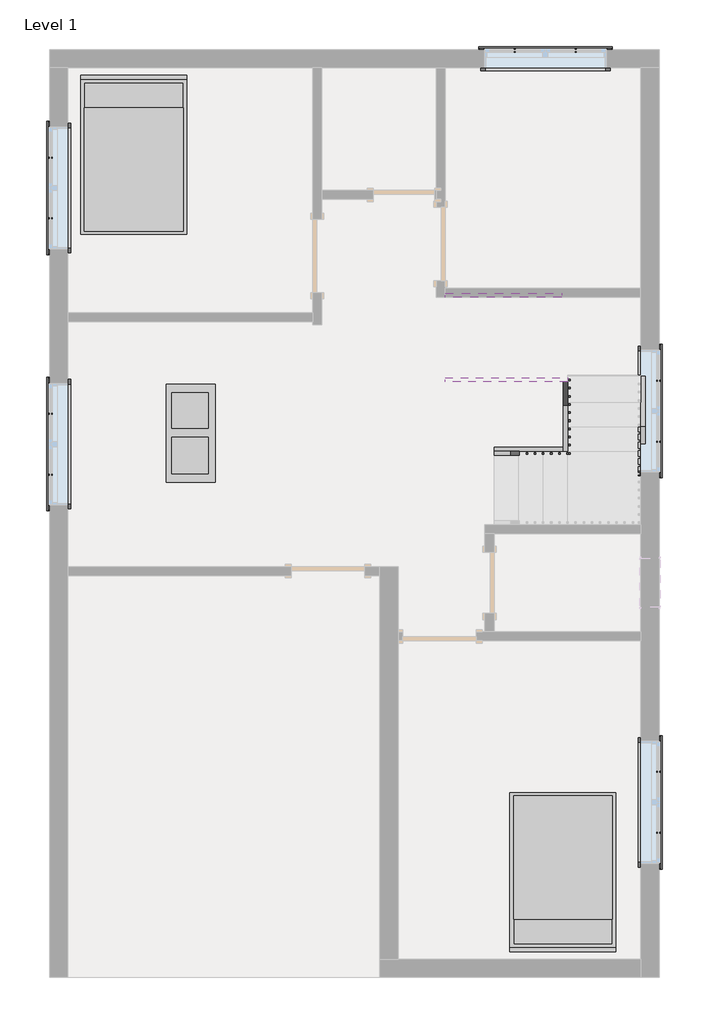
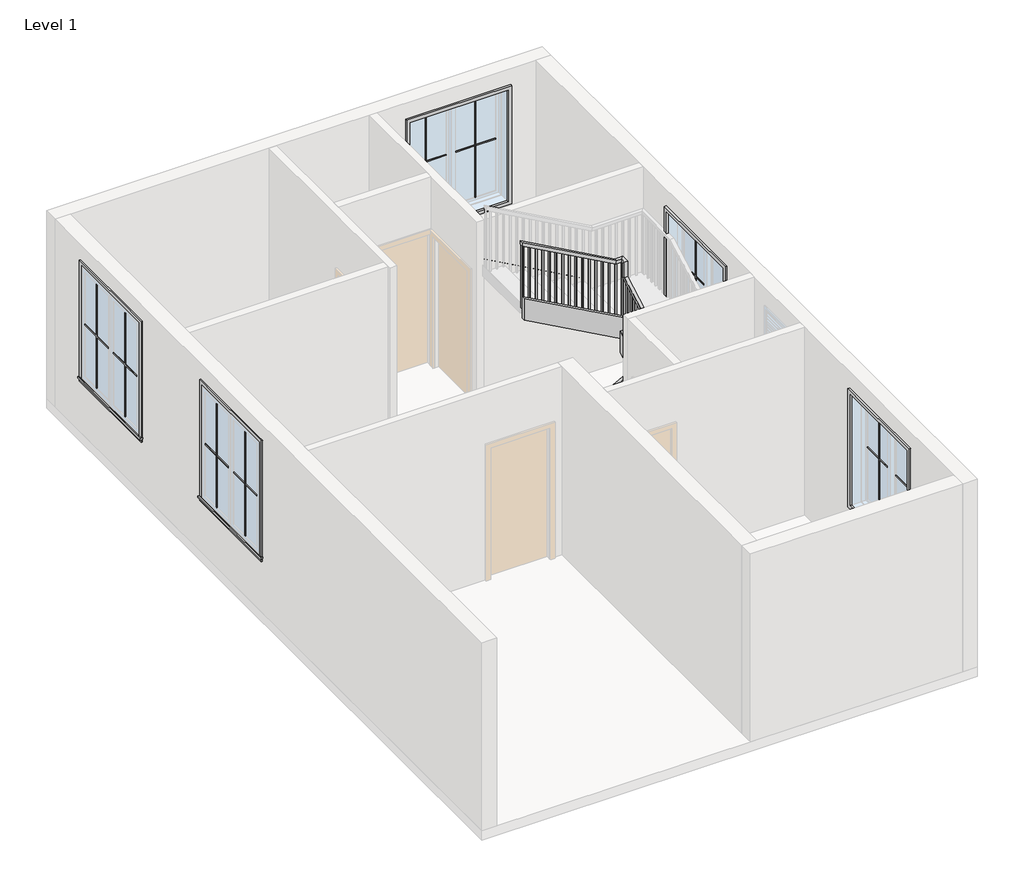
# One storey, part 2 of 2: 21 proxies, 6 members, 2 furniture elements, 1 railing.
"""IFC4 building model written with IfcOpenShell, lengths in millimetres."""

from ifc_helpers import new_model, si_unit, frame, origin, place, context, project, spatial, polyline, outline, extrude, faceted_brep, transform, mapped, element, save
from components import muntin_pattern_2x2_muntin_pattern_2x2_f6a80940, muntin_pattern_2x2_muntin_pattern_2x2_09b00a1c, trim_window_exterior_flat_with_sill_698ed857, trim_window_interior_flat_picture_frame_92551a5e, coffee_table_with_brass_mullions_11320_coffee_table_with_5962bef7, bed_17739_bed_17739_15c61121

model = new_model("IFC4")

# Units and contexts
model_context = context("Model", 3, world=origin())
ifc_project = project(units=[si_unit("LENGTHUNIT", "METRE", prefix="MILLI")], contexts=[model_context])

# Site, building, storey
site = spatial("IfcSite", under=ifc_project)
building = spatial("IfcBuilding", under=site)
storey = spatial("IfcBuildingStorey", under=building, Name="Level 1", Elevation=0.0)

# Proxies
placement = place(None, origin())
muntin_pattern_2x2_muntin_pattern_2x2_shape = muntin_pattern_2x2_muntin_pattern_2x2_f6a80940(model_context)
element("IfcBuildingElementProxy", 1, Name="Muntin Pattern_2x2 : Muntin Pattern_2x2", ObjectType="Muntin Pattern_2x2 : Muntin Pattern_2x2", at=placement, inside=storey, context=model_context, shape_type="MappedRepresentation", body=[
    mapped(muntin_pattern_2x2_muntin_pattern_2x2_shape, transform((-4589.1575206, 441.8004493, 984.25), x_axis=(0.0, 1.0, 0.0), y_axis=(-1.0, 0.0, 0.0), z_axis=(0.0, 0.0, 1.0))),
])
element("IfcBuildingElementProxy", 2, Name="Muntin Pattern_2x2 : Muntin Pattern_2x2", ObjectType="Muntin Pattern_2x2 : Muntin Pattern_2x2", at=placement, inside=storey, context=model_context, shape_type="MappedRepresentation", body=[
    mapped(muntin_pattern_2x2_muntin_pattern_2x2_shape, transform((-4589.1575206, 3632.6754493, 984.25), x_axis=(0.0, 1.0, 0.0), y_axis=(-1.0, 0.0, 0.0), z_axis=(0.0, 0.0, 1.0))),
])
element("IfcBuildingElementProxy", 3, Name="Muntin Pattern_2x2 : Muntin Pattern_2x2", ObjectType="Muntin Pattern_2x2 : Muntin Pattern_2x2", at=placement, inside=storey, context=model_context, shape_type="MappedRepresentation", body=[
    mapped(muntin_pattern_2x2_muntin_pattern_2x2_shape, transform((1197.2799794, 5726.5879493, 984.25), x_axis=(1.0, 0.0, 0.0), y_axis=(0.0, 1.0, 0.0), z_axis=(0.0, 0.0, 1.0))),
])
element("IfcBuildingElementProxy", 4, Name="Muntin Pattern_2x2 : Muntin Pattern_2x2", ObjectType="Muntin Pattern_2x2 : Muntin Pattern_2x2", at=placement, inside=storey, context=model_context, shape_type="MappedRepresentation", body=[
    mapped(muntin_pattern_2x2_muntin_pattern_2x2_shape, transform((2986.3924794, 1613.3754493, 984.25), x_axis=(0.0, -1.0, 0.0), y_axis=(1.0, 0.0, 0.0), z_axis=(0.0, 0.0, 1.0))),
])
element("IfcBuildingElementProxy", 5, Name="Muntin Pattern_2x2 : Muntin Pattern_2x2", ObjectType="Muntin Pattern_2x2 : Muntin Pattern_2x2", at=placement, inside=storey, context=model_context, shape_type="MappedRepresentation", body=[
    mapped(muntin_pattern_2x2_muntin_pattern_2x2_shape, transform((2986.3924794, -3260.2495507, 984.25), x_axis=(0.0, -1.0, 0.0), y_axis=(1.0, 0.0, 0.0), z_axis=(0.0, 0.0, 1.0))),
])
muntin_pattern_2x2_muntin_pattern_2x2_2_shape = muntin_pattern_2x2_muntin_pattern_2x2_09b00a1c(model_context)
element("IfcBuildingElementProxy", 6, Name="Muntin Pattern_2x2 : Muntin Pattern_2x2", ObjectType="Muntin Pattern_2x2 : Muntin Pattern_2x2", at=placement, inside=storey, context=model_context, shape_type="MappedRepresentation", body=[
    mapped(muntin_pattern_2x2_muntin_pattern_2x2_2_shape, transform((-4589.1575206, 1200.6254493, 984.25), x_axis=(0.0, -1.0, 0.0), y_axis=(1.0, 0.0, 0.0), z_axis=(0.0, 0.0, 1.0))),
])
element("IfcBuildingElementProxy", 7, Name="Muntin Pattern_2x2 : Muntin Pattern_2x2", ObjectType="Muntin Pattern_2x2 : Muntin Pattern_2x2", at=placement, inside=storey, context=model_context, shape_type="MappedRepresentation", body=[
    mapped(muntin_pattern_2x2_muntin_pattern_2x2_2_shape, transform((-4589.1575206, 4391.5004493, 984.25), x_axis=(0.0, -1.0, 0.0), y_axis=(1.0, 0.0, 0.0), z_axis=(0.0, 0.0, 1.0))),
])
element("IfcBuildingElementProxy", 8, Name="Muntin Pattern_2x2 : Muntin Pattern_2x2", ObjectType="Muntin Pattern_2x2 : Muntin Pattern_2x2", at=placement, inside=storey, context=model_context, shape_type="MappedRepresentation", body=[
    mapped(muntin_pattern_2x2_muntin_pattern_2x2_2_shape, transform((1956.1049794, 5726.5879493, 984.25), x_axis=(-1.0, 0.0, 0.0), y_axis=(0.0, -1.0, 0.0), z_axis=(0.0, 0.0, 1.0))),
])
element("IfcBuildingElementProxy", 9, Name="Muntin Pattern_2x2 : Muntin Pattern_2x2", ObjectType="Muntin Pattern_2x2 : Muntin Pattern_2x2", at=placement, inside=storey, context=model_context, shape_type="MappedRepresentation", body=[
    mapped(muntin_pattern_2x2_muntin_pattern_2x2_2_shape, transform((2986.3924794, 854.5504493, 984.25), x_axis=(0.0, 1.0, 0.0), y_axis=(-1.0, 0.0, 0.0), z_axis=(0.0, 0.0, 1.0))),
])
element("IfcBuildingElementProxy", 10, Name="Muntin Pattern_2x2 : Muntin Pattern_2x2", ObjectType="Muntin Pattern_2x2 : Muntin Pattern_2x2", at=placement, inside=storey, context=model_context, shape_type="MappedRepresentation", body=[
    mapped(muntin_pattern_2x2_muntin_pattern_2x2_2_shape, transform((2986.3924794, -4019.0745507, 984.25), x_axis=(0.0, 1.0, 0.0), y_axis=(-1.0, 0.0, 0.0), z_axis=(0.0, 0.0, 1.0))),
])
trim_window_exterior_flat_with_sill_shape = trim_window_exterior_flat_with_sill_698ed857(model_context)
element("IfcBuildingElementProxy", 11, Name="Trim-Window-Exterior-Flat : with Sill", ObjectType="Trim-Window-Exterior-Flat : with Sill", at=placement, inside=storey, context=model_context, shape_type="MappedRepresentation", body=[
    mapped(trim_window_exterior_flat_with_sill_shape, transform((-4598.6825206, 821.2129493, 2743.2), x_axis=(0.0, -1.0, 0.0), y_axis=(0.0, 0.0, 1.0), z_axis=(-1.0, 0.0, 0.0))),
])
element("IfcBuildingElementProxy", 12, Name="Trim-Window-Exterior-Flat : with Sill", ObjectType="Trim-Window-Exterior-Flat : with Sill", at=placement, inside=storey, context=model_context, shape_type="MappedRepresentation", body=[
    mapped(trim_window_exterior_flat_with_sill_shape, transform((-4598.6825206, 4012.0879493, 2743.2), x_axis=(0.0, -1.0, 0.0), y_axis=(0.0, 0.0, 1.0), z_axis=(-1.0, 0.0, 0.0))),
])
element("IfcBuildingElementProxy", 13, Name="Trim-Window-Exterior-Flat : with Sill", ObjectType="Trim-Window-Exterior-Flat : with Sill", at=placement, inside=storey, context=model_context, shape_type="MappedRepresentation", body=[
    mapped(trim_window_exterior_flat_with_sill_shape, transform((1576.6924794, 5736.1129493, 2743.2), x_axis=(-1.0, 0.0, 0.0), y_axis=(0.0, 0.0, 1.0), z_axis=(0.0, 1.0, 0.0))),
])
element("IfcBuildingElementProxy", 14, Name="Trim-Window-Exterior-Flat : with Sill", ObjectType="Trim-Window-Exterior-Flat : with Sill", at=placement, inside=storey, context=model_context, shape_type="MappedRepresentation", body=[
    mapped(trim_window_exterior_flat_with_sill_shape, transform((2995.9174794, 1233.9629493, 2743.2), x_axis=(0.0, 1.0, 0.0), y_axis=(0.0, 0.0, 1.0), z_axis=(1.0, 0.0, 0.0))),
])
element("IfcBuildingElementProxy", 15, Name="Trim-Window-Exterior-Flat : with Sill", ObjectType="Trim-Window-Exterior-Flat : with Sill", at=placement, inside=storey, context=model_context, shape_type="MappedRepresentation", body=[
    mapped(trim_window_exterior_flat_with_sill_shape, transform((2995.9174794, -3639.6620507, 2743.2), x_axis=(0.0, 1.0, 0.0), y_axis=(0.0, 0.0, 1.0), z_axis=(1.0, 0.0, 0.0))),
])
trim_window_interior_flat_picture_frame_shape = trim_window_interior_flat_picture_frame_92551a5e(model_context)
element("IfcBuildingElementProxy", 16, Name="Trim-Window-Interior-Flat : Picture Frame", ObjectType="Trim-Window-Interior-Flat : Picture Frame", at=placement, inside=storey, context=model_context, shape_type="MappedRepresentation", body=[
    mapped(trim_window_interior_flat_picture_frame_shape, transform((-4370.0825206, 821.2129493, 2743.2), x_axis=(0.0, 1.0, 0.0), y_axis=(0.0, 0.0, 1.0), z_axis=(1.0, 0.0, 0.0))),
])
element("IfcBuildingElementProxy", 17, Name="Trim-Window-Interior-Flat : Picture Frame", ObjectType="Trim-Window-Interior-Flat : Picture Frame", at=placement, inside=storey, context=model_context, shape_type="MappedRepresentation", body=[
    mapped(trim_window_interior_flat_picture_frame_shape, transform((-4370.0825206, 4012.0879493, 2743.2), x_axis=(0.0, 1.0, 0.0), y_axis=(0.0, 0.0, 1.0), z_axis=(1.0, 0.0, 0.0))),
])
element("IfcBuildingElementProxy", 18, Name="Trim-Window-Interior-Flat : Picture Frame", ObjectType="Trim-Window-Interior-Flat : Picture Frame", at=placement, inside=storey, context=model_context, shape_type="MappedRepresentation", body=[
    mapped(trim_window_interior_flat_picture_frame_shape, transform((1576.6924794, 5507.5129493, 2743.2), x_axis=(1.0, 0.0, 0.0), y_axis=(0.0, 0.0, 1.0), z_axis=(0.0, -1.0, 0.0))),
])
element("IfcBuildingElementProxy", 19, Name="Trim-Window-Interior-Flat : Picture Frame", ObjectType="Trim-Window-Interior-Flat : Picture Frame", at=placement, inside=storey, context=model_context, shape_type="MappedRepresentation", body=[
    mapped(trim_window_interior_flat_picture_frame_shape, transform((2767.3174794, 1233.9629493, 2743.2), x_axis=(0.0, -1.0, 0.0), y_axis=(0.0, 0.0, 1.0), z_axis=(-1.0, 0.0, 0.0))),
])
element("IfcBuildingElementProxy", 20, Name="Trim-Window-Interior-Flat : Picture Frame", ObjectType="Trim-Window-Interior-Flat : Picture Frame", at=placement, inside=storey, context=model_context, shape_type="MappedRepresentation", body=[
    mapped(trim_window_interior_flat_picture_frame_shape, transform((2767.3174794, -3639.6620507, 2743.2), x_axis=(0.0, -1.0, 0.0), y_axis=(0.0, 0.0, 1.0), z_axis=(-1.0, 0.0, 0.0))),
])
coffee_table_with_brass_mullions_11320_coffee_table_with_shape = coffee_table_with_brass_mullions_11320_coffee_table_with_5962bef7(model_context)
element("IfcBuildingElementProxy", 21, Name="coffee_table_with_brass_mullions_11320 : coffee_table_with_brass_mullions_11320", ObjectType="coffee_table_with_brass_mullions_11320 : coffee_table_with_brass_mullions_11320", at=placement, inside=storey, context=model_context, shape_type="MappedRepresentation", body=[
    mapped(coffee_table_with_brass_mullions_11320_coffee_table_with_shape, transform((-2412.0418112, 1596.9678033, 0.0), x_axis=(0.0, 1.0, 0.0), y_axis=(-1.0, 0.0, 0.0), z_axis=(0.0, 0.0, 1.0))),
])

# Furniture
bed_17739_bed_17739_shape = bed_17739_bed_17739_15c61121(model_context)
element("IfcFurniture", 22, ObjectType="Bed_17739 : Bed_17739", at=placement, inside=storey, context=model_context, shape_type="MappedRepresentation", body=[
    mapped(bed_17739_bed_17739_shape, transform((-3550.9325206, 4402.6129493, 0.0), x_axis=(1.0, 0.0, 0.0), y_axis=(0.0, 1.0, 0.0), z_axis=(0.0, 0.0, 1.0))),
])
element("IfcFurniture", 23, ObjectType="Bed_17739 : Bed_17739", at=placement, inside=storey, context=model_context, shape_type="MappedRepresentation", body=[
    mapped(bed_17739_bed_17739_shape, transform((1795.7674794, -4487.3870507, 0.0), x_axis=(-1.0, 0.0, 0.0), y_axis=(0.0, -1.0, 0.0), z_axis=(0.0, 0.0, 1.0))),
])

# Members
element("IfcMember", 24, ObjectType="Stringer - 2\" Width", at=placement, inside=storey, context=model_context, shape_type="SweptSolid", body=[
    extrude(outline(polyline([(207.5983948, 938.5174794), (0.0, 938.5174794), (0.0, 1192.4619822), (338.6974984, 1802.1174794), (687.3761726, 1802.1174794), (207.5983948, 938.5174794)])), frame((0.0, 732.3129493, 0.0), z_axis=(0.0, 1.0, 0.0), x_axis=(0.0, 0.0, 1.0)), (0.0, 0.0, 1.0), 50.8),
])
element("IfcMember", 25, ObjectType="Stringer - 2\" Width", at=placement, inside=storey, context=model_context, shape_type="SweptSolid", body=[
    extrude(outline(polyline([(732.3129493, 536.253054), (732.3129493, 884.9317281), (1595.9129493, 1364.7095059), (1595.9129493, 1016.0308318), (732.3129493, 536.253054)])), frame((1802.1174794, 0.0, 0.0), z_axis=(1.0, 0.0, 0.0), x_axis=(0.0, 1.0, 0.0)), (0.0, 0.0, 1.0), 50.8),
])
element("IfcMember", 26, ObjectType="Stringer - 2\" Width", at=placement, inside=storey, context=model_context, shape_type="SweptSolid", body=[
    extrude(outline(polyline([(1213.5863873, 1852.9174794), (1562.2650614, 1852.9174794), (2408.9317281, 328.9174794), (2060.253054, 328.9174794), (1213.5863873, 1852.9174794)])), frame((0.0, 1595.9129493, 0.0), z_axis=(0.0, 1.0, 0.0), x_axis=(0.0, 0.0, 1.0)), (0.0, 0.0, 1.0), 50.8),
])
element("IfcMember", 27, ObjectType="Stringer - 2\" Width", at=placement, inside=storey, context=model_context, shape_type="SweptSolid", body=[
    extrude(outline(polyline([(207.5983948, 938.5174794), (0.0, 938.5174794), (0.0, 1192.4619822), (376.9317281, 1870.9390928), (376.9317281, 1243.3174794), (207.5983948, 938.5174794)])), frame((0.0, -232.8870507, 0.0), z_axis=(0.0, 1.0, 0.0), x_axis=(0.0, 0.0, 1.0)), (0.0, 0.0, 1.0), 50.8),
])
element("IfcMember", 28, ObjectType="Stringer - 2\" Width", at=placement, inside=storey, context=model_context, shape_type="SweptSolid", body=[
    extrude(outline(polyline([(714.2913359, 874.9197207), (1037.1129493, 1054.2650614), (1664.7345627, 1054.2650614), (1341.9129493, 874.9197207), (714.2913359, 874.9197207)])), frame((2767.3174794, 0.0, 0.0), z_axis=(1.0, 0.0, 0.0), x_axis=(0.0, 1.0, 0.0)), (0.0, 0.0, 1.0), 50.8),
])
element("IfcMember", 29, ObjectType="Stringer - 2\" Width", at=placement, inside=storey, context=model_context, shape_type="SweptSolid", body=[
    extrude(outline(polyline([(1601.6419429, 1782.0390928), (2408.9317281, 328.9174794), (2060.253054, 328.9174794), (1601.6419429, 1154.4174794), (1601.6419429, 1782.0390928)])), frame((0.0, 2650.0129493, 0.0), z_axis=(0.0, 1.0, 0.0), x_axis=(0.0, 0.0, 1.0)), (0.0, 0.0, 1.0), 50.8),
])

# Railing
element("IfcRailing", 30, ObjectType="Handrail - Rectangular", at=placement, inside=storey, context=model_context, shape_type="SolidModel", body=[
    faceted_brep([(938.5174794, 732.3129493, 1083.7333333), (938.5174794, 732.3129493, 1025.620221), (938.5174794, 681.5129493, 1025.620221), (938.5174794, 681.5129493, 1083.7333333), (1776.7174794, 732.3129493, 1549.4), (1827.5174794, 732.3129493, 1519.5091099), (1827.5174794, 681.5129493, 1519.5091099), (1776.7174794, 681.5129493, 1549.4), (1776.7174794, 732.3129493, 1803.4), (1827.5174794, 732.3129493, 1752.6), (1827.5174794, 681.5129493, 1752.6), (1776.7174794, 681.5129493, 1803.4), (1852.9174794, 732.3129493, 1803.4), (1852.9174794, 732.3129493, 1752.6), (1903.7174794, 681.5129493, 1752.6), (1903.7174794, 681.5129493, 1803.4), (1852.9174794, 808.5129493, 1803.4), (1852.9174794, 821.6765516, 1752.6), (1903.7174794, 821.6765516, 1752.6), (1903.7174794, 808.5129493, 1803.4), (1852.9174794, 1570.5129493, 2226.7333333), (1852.9174794, 1621.3129493, 2196.8424432), (1903.7174794, 1621.3129493, 2196.8424432), (1903.7174794, 1570.5129493, 2226.7333333), (1852.9174794, 1570.5129493, 2480.7333333), (1852.9174794, 1621.3129493, 2429.9333333), (1903.7174794, 1621.3129493, 2429.9333333), (1903.7174794, 1570.5129493, 2480.7333333), (1852.9174794, 1646.7129493, 2480.7333333), (1852.9174794, 1646.7129493, 2429.9333333), (1903.7174794, 1697.5129493, 2429.9333333), (1903.7174794, 1697.5129493, 2480.7333333), (1776.7174794, 1646.7129493, 2480.7333333), (1763.5538772, 1646.7129493, 2429.9333333), (1763.5538772, 1697.5129493, 2429.9333333), (1776.7174794, 1697.5129493, 2480.7333333), (328.9174794, 1646.7129493, 3285.0666667), (328.9174794, 1697.5129493, 3285.0666667), (328.9174794, 1697.5129493, 3226.9535543), (328.9174794, 1646.7129493, 3226.9535543)], [[[0, 1, 2, 3]], [[1, 0, 4, 5]], [[2, 1, 5, 6]], [[3, 2, 6, 7]], [[0, 3, 7, 4]], [[5, 4, 8, 9]], [[6, 5, 9, 10]], [[7, 6, 10, 11]], [[4, 7, 11, 8]], [[9, 8, 12, 13]], [[10, 9, 13, 14]], [[11, 10, 14, 15]], [[8, 11, 15, 12]], [[13, 12, 16, 17]], [[14, 13, 17, 18]], [[15, 14, 18, 19]], [[12, 15, 19, 16]], [[17, 16, 20, 21]], [[18, 17, 21, 22]], [[19, 18, 22, 23]], [[16, 19, 23, 20]], [[21, 20, 24, 25]], [[22, 21, 25, 26]], [[23, 22, 26, 27]], [[20, 23, 27, 24]], [[25, 24, 28, 29]], [[26, 25, 29, 30]], [[27, 26, 30, 31]], [[24, 27, 31, 28]], [[29, 28, 32, 33]], [[30, 29, 33, 34]], [[31, 30, 34, 35]], [[28, 31, 35, 32]], [[36, 37, 38, 39]], [[33, 32, 36, 39]], [[34, 33, 39, 38]], [[35, 34, 38, 37]], [[32, 35, 37, 36]]]),
    extrude(outline(polyline([(3218.1341099, 344.7924794), (2201.3333333, 344.7924794), (2201.3333333, 363.8424794), (3207.5507765, 363.8424794), (3218.1341099, 344.7924794)])), frame((0.0, 1662.5879493, 0.0), z_axis=(0.0, 1.0, 0.0), x_axis=(0.0, 0.0, 1.0)), (0.0, 0.0, 1.0), 19.05),
    extrude(outline(polyline([(3161.6896654, 446.3924794), (2201.3333333, 446.3924794), (2201.3333333, 465.4424794), (3151.1063321, 465.4424794), (3161.6896654, 446.3924794)])), frame((0.0, 1662.5879493, 0.0), z_axis=(0.0, 1.0, 0.0), x_axis=(0.0, 0.0, 1.0)), (0.0, 0.0, 1.0), 19.05),
    extrude(outline(polyline([(3105.245221, 547.9924794), (2201.3333333, 547.9924794), (2201.3333333, 567.0424794), (3094.6618876, 567.0424794), (3105.245221, 547.9924794)])), frame((0.0, 1662.5879493, 0.0), z_axis=(0.0, 1.0, 0.0), x_axis=(0.0, 0.0, 1.0)), (0.0, 0.0, 1.0), 19.05),
    extrude(outline(polyline([(3048.8007765, 649.5924794), (2032.0, 649.5924794), (2032.0, 668.6424794), (3038.2174432, 668.6424794), (3048.8007765, 649.5924794)])), frame((0.0, 1662.5879493, 0.0), z_axis=(0.0, 1.0, 0.0), x_axis=(0.0, 0.0, 1.0)), (0.0, 0.0, 1.0), 19.05),
    extrude(outline(polyline([(2992.3563321, 751.1924794), (2032.0, 751.1924794), (2032.0, 770.2424794), (2981.7729988, 770.2424794), (2992.3563321, 751.1924794)])), frame((0.0, 1662.5879493, 0.0), z_axis=(0.0, 1.0, 0.0), x_axis=(0.0, 0.0, 1.0)), (0.0, 0.0, 1.0), 19.05),
    extrude(outline(polyline([(2935.9118876, 852.7924794), (2032.0, 852.7924794), (2032.0, 871.8424794), (2925.3285543, 871.8424794), (2935.9118876, 852.7924794)])), frame((0.0, 1662.5879493, 0.0), z_axis=(0.0, 1.0, 0.0), x_axis=(0.0, 0.0, 1.0)), (0.0, 0.0, 1.0), 19.05),
    extrude(outline(polyline([(2879.4674432, 954.3924794), (1862.6666667, 954.3924794), (1862.6666667, 973.4424794), (2868.8841099, 973.4424794), (2879.4674432, 954.3924794)])), frame((0.0, 1662.5879493, 0.0), z_axis=(0.0, 1.0, 0.0), x_axis=(0.0, 0.0, 1.0)), (0.0, 0.0, 1.0), 19.05),
    extrude(outline(polyline([(2823.0229988, 1055.9924794), (1862.6666667, 1055.9924794), (1862.6666667, 1075.0424794), (2812.4396654, 1075.0424794), (2823.0229988, 1055.9924794)])), frame((0.0, 1662.5879493, 0.0), z_axis=(0.0, 1.0, 0.0), x_axis=(0.0, 0.0, 1.0)), (0.0, 0.0, 1.0), 19.05),
    extrude(outline(polyline([(2766.5785543, 1157.5924794), (1862.6666667, 1157.5924794), (1862.6666667, 1176.6424794), (2755.995221, 1176.6424794), (2766.5785543, 1157.5924794)])), frame((0.0, 1662.5879493, 0.0), z_axis=(0.0, 1.0, 0.0), x_axis=(0.0, 0.0, 1.0)), (0.0, 0.0, 1.0), 19.05),
    extrude(outline(polyline([(2710.1341099, 1259.1924794), (1693.3333333, 1259.1924794), (1693.3333333, 1278.2424794), (2699.5507765, 1278.2424794), (2710.1341099, 1259.1924794)])), frame((0.0, 1662.5879493, 0.0), z_axis=(0.0, 1.0, 0.0), x_axis=(0.0, 0.0, 1.0)), (0.0, 0.0, 1.0), 19.05),
    extrude(outline(polyline([(2653.6896654, 1360.7924794), (1693.3333333, 1360.7924794), (1693.3333333, 1379.8424794), (2643.1063321, 1379.8424794), (2653.6896654, 1360.7924794)])), frame((0.0, 1662.5879493, 0.0), z_axis=(0.0, 1.0, 0.0), x_axis=(0.0, 0.0, 1.0)), (0.0, 0.0, 1.0), 19.05),
    extrude(outline(polyline([(2597.245221, 1462.3924794), (1693.3333333, 1462.3924794), (1693.3333333, 1481.4424794), (2586.6618876, 1481.4424794), (2597.245221, 1462.3924794)])), frame((0.0, 1662.5879493, 0.0), z_axis=(0.0, 1.0, 0.0), x_axis=(0.0, 0.0, 1.0)), (0.0, 0.0, 1.0), 19.05),
    extrude(outline(polyline([(2540.8007765, 1563.9924794), (1524.0, 1563.9924794), (1524.0, 1583.0424794), (2530.2174432, 1583.0424794), (2540.8007765, 1563.9924794)])), frame((0.0, 1662.5879493, 0.0), z_axis=(0.0, 1.0, 0.0), x_axis=(0.0, 0.0, 1.0)), (0.0, 0.0, 1.0), 19.05),
    extrude(outline(polyline([(2484.3563321, 1665.5924794), (1524.0, 1665.5924794), (1524.0, 1684.6424794), (2473.7729988, 1684.6424794), (2484.3563321, 1665.5924794)])), frame((0.0, 1662.5879493, 0.0), z_axis=(0.0, 1.0, 0.0), x_axis=(0.0, 0.0, 1.0)), (0.0, 0.0, 1.0), 19.05),
    extrude(outline(polyline([(2427.9118876, 1767.1924794), (1524.0, 1767.1924794), (1524.0, 1786.2424794), (2417.3285543, 1786.2424794), (2427.9118876, 1767.1924794)])), frame((0.0, 1662.5879493, 0.0), z_axis=(0.0, 1.0, 0.0), x_axis=(0.0, 0.0, 1.0)), (0.0, 0.0, 1.0), 19.05),
    extrude(outline(polyline([(1868.7924794, 1611.7879493), (1868.7924794, 1630.8379493), (1887.8424794, 1630.8379493), (1887.8424794, 1611.7879493), (1868.7924794, 1611.7879493)])), frame((0.0, 0.0, 1185.3333333), z_axis=(0.0, 0.0, 1.0), x_axis=(1.0, 0.0, 0.0)), (0.0, 0.0, 1.0), 1244.6),
    extrude(outline(polyline([(1529.2379493, 2145.6896654), (1529.2379493, 1185.3333333), (1510.1879493, 1185.3333333), (1510.1879493, 2135.1063321), (1529.2379493, 2145.6896654)])), frame((1868.7924794, 0.0, 0.0), z_axis=(1.0, 0.0, 0.0), x_axis=(0.0, 1.0, 0.0)), (0.0, 0.0, 1.0), 19.05),
    extrude(outline(polyline([(1427.6379493, 2089.245221), (1427.6379493, 1185.3333333), (1408.5879493, 1185.3333333), (1408.5879493, 2078.6618876), (1427.6379493, 2089.245221)])), frame((1868.7924794, 0.0, 0.0), z_axis=(1.0, 0.0, 0.0), x_axis=(0.0, 1.0, 0.0)), (0.0, 0.0, 1.0), 19.05),
    extrude(outline(polyline([(1326.0379493, 2032.8007765), (1326.0379493, 1016.0), (1306.9879493, 1016.0), (1306.9879493, 2022.2174432), (1326.0379493, 2032.8007765)])), frame((1868.7924794, 0.0, 0.0), z_axis=(1.0, 0.0, 0.0), x_axis=(0.0, 1.0, 0.0)), (0.0, 0.0, 1.0), 19.05),
    extrude(outline(polyline([(1224.4379493, 1976.3563321), (1224.4379493, 1016.0), (1205.3879493, 1016.0), (1205.3879493, 1965.7729988), (1224.4379493, 1976.3563321)])), frame((1868.7924794, 0.0, 0.0), z_axis=(1.0, 0.0, 0.0), x_axis=(0.0, 1.0, 0.0)), (0.0, 0.0, 1.0), 19.05),
    extrude(outline(polyline([(1122.8379493, 1919.9118876), (1122.8379493, 1016.0), (1103.7879493, 1016.0), (1103.7879493, 1909.3285543), (1122.8379493, 1919.9118876)])), frame((1868.7924794, 0.0, 0.0), z_axis=(1.0, 0.0, 0.0), x_axis=(0.0, 1.0, 0.0)), (0.0, 0.0, 1.0), 19.05),
    extrude(outline(polyline([(1021.2379493, 1863.4674432), (1021.2379493, 846.6666667), (1002.1879493, 846.6666667), (1002.1879493, 1852.8841099), (1021.2379493, 1863.4674432)])), frame((1868.7924794, 0.0, 0.0), z_axis=(1.0, 0.0, 0.0), x_axis=(0.0, 1.0, 0.0)), (0.0, 0.0, 1.0), 19.05),
    extrude(outline(polyline([(919.6379493, 1807.0229988), (919.6379493, 846.6666667), (900.5879493, 846.6666667), (900.5879493, 1796.4396654), (919.6379493, 1807.0229988)])), frame((1868.7924794, 0.0, 0.0), z_axis=(1.0, 0.0, 0.0), x_axis=(0.0, 1.0, 0.0)), (0.0, 0.0, 1.0), 19.05),
    extrude(outline(polyline([(818.0379493, 1750.5785543), (818.0379493, 846.6666667), (798.9879493, 846.6666667), (798.9879493, 1739.995221), (818.0379493, 1750.5785543)])), frame((1868.7924794, 0.0, 0.0), z_axis=(1.0, 0.0, 0.0), x_axis=(0.0, 1.0, 0.0)), (0.0, 0.0, 1.0), 19.05),
    extrude(outline(polyline([(1843.3924794, 716.4379493), (1862.4424794, 716.4379493), (1862.4424794, 697.3879493), (1843.3924794, 697.3879493), (1843.3924794, 716.4379493)])), frame((0.0, 0.0, 677.3333333), z_axis=(0.0, 0.0, 1.0), x_axis=(1.0, 0.0, 0.0)), (0.0, 0.0, 1.0), 1075.2666667),
    extrude(outline(polyline([(1471.8841099, 1741.7924794), (508.0, 1741.7924794), (508.0, 1760.8424794), (1482.4674432, 1760.8424794), (1471.8841099, 1741.7924794)])), frame((0.0, 697.3879493, 0.0), z_axis=(0.0, 1.0, 0.0), x_axis=(0.0, 0.0, 1.0)), (0.0, 0.0, 1.0), 19.05),
    extrude(outline(polyline([(1415.4396654, 1640.1924794), (508.0, 1640.1924794), (508.0, 1659.2424794), (1426.0229988, 1659.2424794), (1415.4396654, 1640.1924794)])), frame((0.0, 697.3879493, 0.0), z_axis=(0.0, 1.0, 0.0), x_axis=(0.0, 0.0, 1.0)), (0.0, 0.0, 1.0), 19.05),
    extrude(outline(polyline([(1358.995221, 1538.5924794), (508.0, 1538.5924794), (508.0, 1557.6424794), (1369.5785543, 1557.6424794), (1358.995221, 1538.5924794)])), frame((0.0, 697.3879493, 0.0), z_axis=(0.0, 1.0, 0.0), x_axis=(0.0, 0.0, 1.0)), (0.0, 0.0, 1.0), 19.05),
    extrude(outline(polyline([(1302.5507765, 1436.9924794), (338.6666667, 1436.9924794), (338.6666667, 1456.0424794), (1313.1341099, 1456.0424794), (1302.5507765, 1436.9924794)])), frame((0.0, 697.3879493, 0.0), z_axis=(0.0, 1.0, 0.0), x_axis=(0.0, 0.0, 1.0)), (0.0, 0.0, 1.0), 19.05),
    extrude(outline(polyline([(1246.1063321, 1335.3924794), (338.6666667, 1335.3924794), (338.6666667, 1354.4424794), (1256.6896654, 1354.4424794), (1246.1063321, 1335.3924794)])), frame((0.0, 697.3879493, 0.0), z_axis=(0.0, 1.0, 0.0), x_axis=(0.0, 0.0, 1.0)), (0.0, 0.0, 1.0), 19.05),
    extrude(outline(polyline([(1189.6618876, 1233.7924794), (338.6666667, 1233.7924794), (338.6666667, 1252.8424794), (1200.245221, 1252.8424794), (1189.6618876, 1233.7924794)])), frame((0.0, 697.3879493, 0.0), z_axis=(0.0, 1.0, 0.0), x_axis=(0.0, 0.0, 1.0)), (0.0, 0.0, 1.0), 19.05),
    extrude(outline(polyline([(1133.2174432, 1132.1924794), (169.3333333, 1132.1924794), (169.3333333, 1151.2424794), (1143.8007765, 1151.2424794), (1133.2174432, 1132.1924794)])), frame((0.0, 697.3879493, 0.0), z_axis=(0.0, 1.0, 0.0), x_axis=(0.0, 0.0, 1.0)), (0.0, 0.0, 1.0), 19.05),
    extrude(outline(polyline([(1076.7729988, 1030.5924794), (169.3333333, 1030.5924794), (169.3333333, 1049.6424794), (1087.3563321, 1049.6424794), (1076.7729988, 1030.5924794)])), frame((0.0, 697.3879493, 0.0), z_axis=(0.0, 1.0, 0.0), x_axis=(0.0, 0.0, 1.0)), (0.0, 0.0, 1.0), 19.05),
    extrude(outline(polyline([(1868.7924794, 1662.5879493), (1868.7924794, 1681.6379493), (1887.8424794, 1681.6379493), (1887.8424794, 1662.5879493), (1868.7924794, 1662.5879493)])), frame((0.0, 0.0, 1354.6666667), z_axis=(0.0, 0.0, 1.0), x_axis=(1.0, 0.0, 0.0)), (0.0, 0.0, 1.0), 1075.2666667),
    extrude(outline(polyline([(1868.7924794, 716.4379493), (1887.8424794, 716.4379493), (1887.8424794, 697.3879493), (1868.7924794, 697.3879493), (1868.7924794, 716.4379493)])), frame((0.0, 0.0, 677.3333333), z_axis=(0.0, 0.0, 1.0), x_axis=(1.0, 0.0, 0.0)), (0.0, 0.0, 1.0), 1075.2666667),
    extrude(outline(polyline([(3226.9535543, 328.9174794), (2201.3333333, 328.9174794), (2201.3333333, 347.9674794), (3216.370221, 347.9674794), (3226.9535543, 328.9174794)])), frame((0.0, 1662.5879493, 0.0), z_axis=(0.0, 1.0, 0.0), x_axis=(0.0, 0.0, 1.0)), (0.0, 0.0, 1.0), 19.05),
    extrude(outline(polyline([(1025.620221, 938.5174794), (169.3333333, 938.5174794), (169.3333333, 957.5674794), (1036.2035543, 957.5674794), (1025.620221, 938.5174794)])), frame((0.0, 697.3879493, 0.0), z_axis=(0.0, 1.0, 0.0), x_axis=(0.0, 0.0, 1.0)), (0.0, 0.0, 1.0), 19.05),
])

save(model, "model.ifc")

# Revit data of these elements
# Type "Muntin Pattern_2x2 : Muntin Pattern_2x2"
#   Width [instance default] = 4' - 0"
#   Thickness = 0' - 0 1/2"
#   Height [instance default] = 4' - 0"
#   Distance = 0' - 0 3/4"
#   Interior Material [instance default] = none
#   Exterior Material [instance default] = none
#   Default Elevation = 0
# Type "Trim-Window-Exterior-Flat : with Sill"
#   Trim Width = 0' - 2 1/4"
#   Trim Thickness_Picture Frame = 0' - 1 1/4"
#   Trim Thickness_with Sill = 0' - 0 3/4"
#   Sill Thickness = 0' - 1 1/4"
#   Opening Width [instance default] = 2' - 0"
#   Opening Height [instance default] = 3' - 0"
#   Default Elevation = 4' - 0"
#   Sill = yes
#   Picture Frame = no
#   Trim Material [instance default] = none
# Type "Trim-Window-Interior-Flat : Picture Frame"
#   Trim Thickness_Picture Frame = 0' - 1 1/4"
#   Trim Width = 0' - 2 1/4"
#   Trim Thickness_with Sill = 0' - 0 3/4"
#   Sill Thickness = 0' - 1 1/4"
#   Opening Width [instance default] = 2' - 0"
#   Opening Height [instance default] = 3' - 0"
#   Default Elevation = 4' - 0"
#   Sill = no
#   Picture Frame = yes
#   Trim Material [instance default] = none
# Type "coffee_table_with_brass_mullions_11320 : coffee_table_with_brass_mullions_11320"
#   Default Elevation = 0
# Type "Bed_17739 : Bed_17739"
#   Default Elevation = 0
# Type "Handrail - Rectangular"
#   Assembly Code = "C2010400"
#   built-in parameter 1008612 = 0.0416667 (stored number, unit not read)
#   built-in parameter 1008611 = 0.0416667 (stored number, unit not read)
#   built-in parameter 1008609 = 0.333333 (stored number, unit not read)
#   built-in parameter 1008604 = 0.166667 (stored number, unit not read)
#   built-in parameter 1008603 = 0.166667 (stored number, unit not read)
#   Railing Height = 3' - 0"
#   built-in parameter 1008630 = 2
#   built-in parameter 1008610 = 2
#   built-in parameter 1008618 = Baluster - Square : 3/4"
# Elements 1, 2, 3, 4, 5, 6, 7, 8, 9, 10 (IfcBuildingElementProxy, "Muntin Pattern_2x2 : Muntin Pattern_2x2")
#   Width = 2' - 0 5/8"
#   Height = 5' - 6 1/2"
#   Interior Material = Wood - Stained
#   Exterior Material = Clad - White
#   Phase Created = New Construction
#   Materials on its faces: "Clad - White", "Wood - Stained"
# Elements 11, 12, 13, 14, 15 (IfcBuildingElementProxy, "Trim-Window-Exterior-Flat : with Sill")
#   Opening Width = 5' - 0"
#   Opening Height = 6' - 0"
#   Trim Material = Clad - White
#   Phase Created = New Construction
#   Materials on its faces: "Clad - White"
# Elements 16, 17, 18, 19, 20 (IfcBuildingElementProxy, "Trim-Window-Interior-Flat : Picture Frame")
#   Opening Width = 5' - 0"
#   Opening Height = 6' - 0"
#   Trim Material = Wood - Stained
#   Phase Created = New Construction
#   Materials on its faces: "Wood - Stained"
# Element 21 (IfcBuildingElementProxy, "coffee_table_with_brass_mullions_11320 : coffee_table_with_brass_mullions_11320")
#   Phase Created = New Construction
#   Materials on its faces: "Default Wall", "TABLE", "Glass", "Default"
# Elements 22, 23 (IfcFurniture, "Bed_17739 : Bed_17739")
#   Phase Created = New Construction
#   Materials on its faces: "legs", "sheets", "bed frame", "Blanket"
# Elements 24, 25, 26, 27, 28, 29 (IfcMember, "Stringer - 2\" Width")
#   Phase Created = New Construction
# Element 30 (IfcRailing, "Handrail - Rectangular")
#   Phase Created = New Construction
# Materials
#   "Clad - White": class "Wood", colour RGB 242 242 238, transparency 0, Cost = 0
#   "Wood - Stained": class "Wood", colour RGB 224 178 126, transparency 0, Cost = 0
#   "Default Wall": colour RGB 128 128 128, transparency 0, Cost = 0
#   "TABLE": class "Generic", colour RGB 120 120 120, transparency 0, Cost = 0
#   "Glass": class "Glass", colour RGB 0 128 192, transparency 0.75, Description = "Soda Lime Glass", Cost = 0
#   "Default": colour RGB 127 127 127, transparency 0, Cost = 0
#   "legs": colour RGB 90 73 37, transparency 0, Cost = 0
#   "sheets": colour RGB 200 195 176, transparency 0, Cost = 0
#   "bed frame": colour RGB 90 73 37, transparency 0, Cost = 0
#   "Blanket": class "System", colour RGB 59 0 1, transparency 0, Cost = 0
